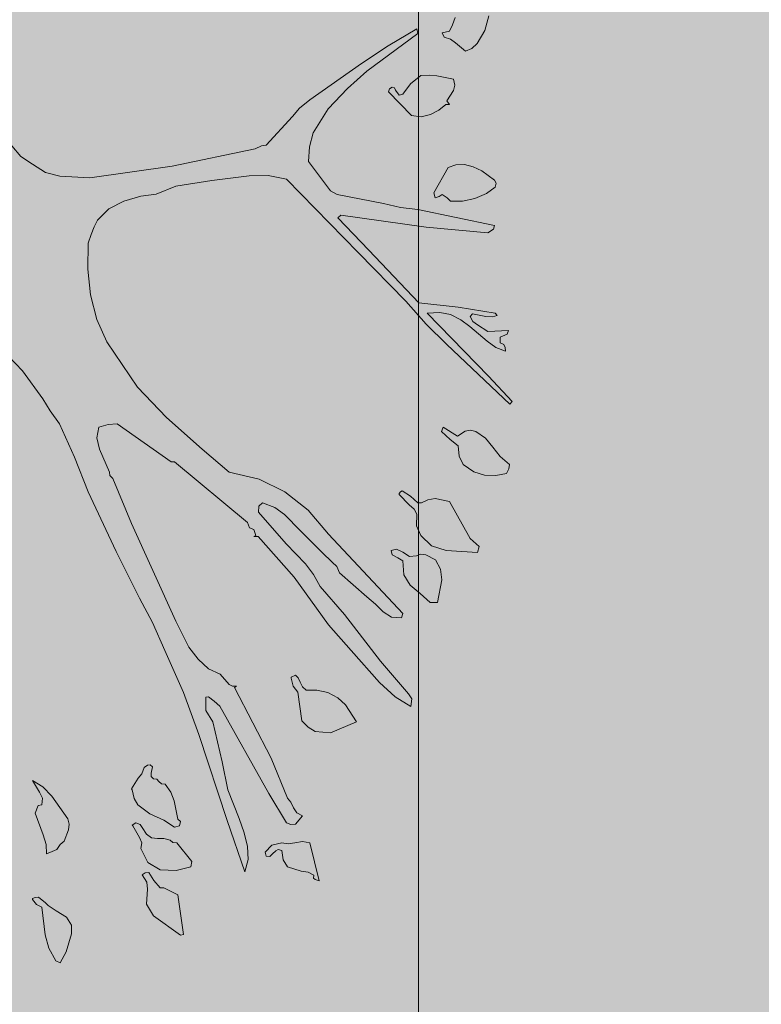
# Model space of a CAD drawing. Units: inches. Extents: x 84 to 1044, y -280 to 906.
# Tile 61 of 105: x 427 to 440, y 731 to 748. Entities that reach past the tile are written whole.
import ezdxf

# ---------------------------------------------------------------- set-up
doc = ezdxf.new("R2010")
doc.units = ezdxf.units.IN
for name, color, linetype, lineweight in [('A-ANNO-DIMS', 2, 'Continuous', 18), ('L-HRDS', 32, 'Continuous', 18), ('L-PLNT', 114, 'Continuous', 15)]:
    doc.layers.add(name, color=color, linetype=linetype, lineweight=lineweight)
doc.layers.add('L-PLNT-PATT', color=9, linetype='Continuous', lineweight=9, true_color=0xafd9aa)
doc.styles.get("Standard").update_dxf_attribs({"font": 'arial.ttf'})
doc.dimstyles.get("Standard").update_dxf_attribs({"dimtxt": 0.18, "dimasz": 0.18, "dimexe": 0.18, "dimexo": 0.0625, "dimgap": 0.09, "dimtad": 0, "dimtih": 1, "dimtoh": 1, "dimdec": 4, "dimzin": 0, "dimdsep": 46, "dimtxsty": 'Standard', "dimcen": 0.09, "dimadec": 0, "dimazin": 0, "dimtfac": 1, "dimtdec": 4, "dimtofl": 0, "dimtmove": 0, "dimatfit": 3, "dimfxl": 1, "dimtolj": 1, "dimtzin": 0, "dimarcsym": 0})

# ---------------------------------------------------------------- blocks, each defined once
blk = doc.blocks.new('A$C37E508DF')
for p, q in [((1.3455, 1.0934), (1.3485, 1.102)), ((1.3875, 1.1037), (1.3828, 1.087)), ((1.2713, 1.0694), (1.3044, 1.0887)), ((1.3044, 1.0887), (1.3057, 1.0835)), ((1.3421, 1.0861), (1.3455, 1.0934)), ((1.3057, 1.0835), (1.2469, 1.0402)), ((1.3335, 1.0844), (1.3421, 1.0861)), ((1.3361, 1.0793), (1.3335, 1.0844)), ((1.3434, 1.0771), (1.3361, 1.0793)), ((1.349, 1.0728), (1.3434, 1.0771)), ((1.3828, 1.087), (1.3738, 1.072)), ((1.2409, 1.0488), (1.2713, 1.0694)), ((1.3605, 1.063), (1.349, 1.0728)), ((1.3678, 1.0664), (1.3605, 1.063)), ((1.3738, 1.072), (1.3678, 1.0664)), ((1.1813, 1.0072), (1.2409, 1.0488)), ((1.2469, 1.0402), (1.2246, 1.0201)), ((1.2971, 1.0257), (1.3091, 1.0351)), ((1.3091, 1.0351), (1.3185, 1.0355)), ((1.3185, 1.0355), (1.3275, 1.0347)), ((1.3275, 1.0347), (1.3468, 1.0308)), ((1.2731, 1.0197), (1.2761, 1.0218)), ((1.2761, 1.0218), (1.2786, 1.0209)), ((1.2786, 1.0209), (1.2799, 1.0184)), ((1.2885, 1.0136), (1.2971, 1.0257)), ((1.3468, 1.0308), (1.3481, 1.0239)), ((1.3481, 1.0239), (1.3468, 1.018)), ((1.2246, 1.0201), (1.2023, 0.9969)), ((1.2718, 1.0162), (1.2731, 1.0197)), ((1.2984, 0.9892), (1.2718, 1.0162)), ((1.2799, 1.0184), (1.2842, 1.0124)), ((1.2842, 1.0124), (1.2885, 1.0136)), ((1.3468, 1.018), (1.3391, 1.0059)), ((1.1693, 0.9974), (1.1813, 1.0072)), ((1.3378, 1.0016), (1.3297, 0.9952)), ((1.3421, 1.0016), (1.3378, 1.0016)), ((1.3391, 1.0059), (1.3421, 1.0016)), ((1.1311, 0.9549), (1.1612, 0.9879)), ((1.1612, 0.9879), (1.1693, 0.9974)), ((1.2023, 0.9969), (1.1852, 0.9691)), ((1.3095, 0.9875), (1.2984, 0.9892)), ((1.3202, 0.9901), (1.3095, 0.9875)), ((1.3297, 0.9952), (1.3202, 0.9901)), ((1.1852, 0.9691), (1.1809, 0.9532)), ((0.8383, 0.954), (0.8486, 0.942)), ((1.1183, 0.9506), (1.1256, 0.954)), ((1.1256, 0.954), (1.1311, 0.9549)), ((1.1809, 0.9532), (1.1796, 0.936)), ((0.8486, 0.942), (0.8619, 0.933)), ((1.0227, 0.9309), (1.1183, 0.9506)), ((0.8619, 0.933), (0.8769, 0.9236)), ((0.9279, 0.9172), (1.0227, 0.9309)), ((1.1796, 0.936), (1.2049, 0.9022)), ((1.3404, 0.9292), (1.3494, 0.9322)), ((1.3494, 0.9322), (1.3592, 0.9326)), ((1.3592, 0.9326), (1.3695, 0.93)), ((1.3695, 0.93), (1.3794, 0.9253)), ((0.8769, 0.9236), (0.8936, 0.9193)), ((0.8936, 0.9193), (0.9279, 0.9172)), ((1.1114, 0.9198), (1.0685, 0.9142)), ((1.1333, 0.9202), (1.1114, 0.9198)), ((1.1543, 0.9159), (1.1333, 0.9202)), ((1.3241, 0.9), (1.3404, 0.9292)), ((1.3794, 0.9253), (1.394, 0.9146)), ((1.0269, 0.9077), (1.0042, 0.8987)), ((1.0685, 0.9142), (1.0269, 0.9077)), ((1.2371, 0.8314), (1.1543, 0.9159)), ((1.394, 0.9146), (1.3957, 0.9112)), ((1.3957, 0.9112), (1.3948, 0.9065)), ((0.9866, 0.8962), (0.9673, 0.8906)), ((1.0042, 0.8987), (0.9866, 0.8962)), ((1.2049, 0.9022), (1.2126, 0.8983)), ((1.2126, 0.8983), (1.2662, 0.8876)), ((1.3254, 0.8944), (1.3241, 0.9)), ((1.3301, 0.8957), (1.3254, 0.8944)), ((1.3335, 0.8983), (1.3301, 0.8957)), ((1.3395, 0.8944), (1.3335, 0.8983)), ((1.3846, 0.8992), (1.3713, 0.8936)), ((1.3948, 0.9065), (1.3846, 0.8992)), ((0.9673, 0.8906), (0.9498, 0.8816)), ((1.2662, 0.8876), (1.2855, 0.8833)), ((1.3434, 0.8906), (1.3395, 0.8944)), ((1.3571, 0.8906), (1.3434, 0.8906)), ((1.3713, 0.8936), (1.3571, 0.8906)), ((0.9498, 0.8816), (0.9369, 0.8687)), ((1.2169, 0.8743), (1.2135, 0.8713)), ((1.3151, 0.8606), (1.2169, 0.8743)), ((1.2855, 0.8833), (1.3057, 0.8807)), ((1.3057, 0.8807), (1.394, 0.8623)), ((0.9369, 0.8687), (0.933, 0.861)), ((1.2135, 0.8713), (1.2491, 0.834)), ((1.394, 0.8623), (1.3927, 0.8584)), ((0.9296, 0.852), (0.9262, 0.8421)), ((0.933, 0.861), (0.9296, 0.852)), ((1.3863, 0.8541), (1.3151, 0.8606)), ((1.3927, 0.8584), (1.3863, 0.8541)), ((0.9262, 0.8421), (0.9257, 0.8121)), ((1.2919, 0.7752), (1.2371, 0.8314)), ((1.2491, 0.834), (1.3069, 0.7735)), ((0.9257, 0.8121), (0.9287, 0.7825)), ((0.9287, 0.7825), (0.936, 0.7542)), ((1.3151, 0.7487), (1.2919, 0.7752)), ((1.3069, 0.7735), (1.352, 0.7684)), ((1.3309, 0.7624), (1.3164, 0.7615)), ((1.3164, 0.7615), (1.3871, 0.6891)), ((1.3434, 0.7598), (1.3309, 0.7624)), ((1.355, 0.7538), (1.3434, 0.7598)), ((1.352, 0.7684), (1.3948, 0.7615)), ((1.3687, 0.7607), (1.3657, 0.7577)), ((1.3841, 0.7577), (1.3687, 0.7607)), ((1.3948, 0.7615), (1.397, 0.759)), ((0.936, 0.7542), (0.9476, 0.7285)), ((1.3391, 0.7255), (1.3151, 0.7487)), ((1.3653, 0.7461), (1.355, 0.7538)), ((1.3657, 0.7577), (1.3691, 0.7521)), ((1.3691, 0.7521), (1.3743, 0.7482)), ((1.3743, 0.7482), (1.3863, 0.7405)), ((1.3914, 0.7572), (1.3841, 0.7577)), ((1.397, 0.759), (1.3914, 0.7572)), ((1.3854, 0.7294), (1.3653, 0.7461)), ((1.3863, 0.7405), (1.4099, 0.7414)), ((1.4086, 0.7375), (1.4004, 0.7337)), ((1.4099, 0.7414), (1.4086, 0.7375)), ((0.9476, 0.7285), (0.9828, 0.6762)), ((1.4116, 0.6569), (1.3391, 0.7255)), ((1.3953, 0.7221), (1.3854, 0.7294)), ((1.4004, 0.7337), (1.4004, 0.7272)), ((1.4004, 0.7272), (1.4047, 0.7255)), ((1.4047, 0.7255), (1.406, 0.7221)), ((1.4064, 0.7178), (1.3953, 0.7221)), ((1.406, 0.7221), (1.4064, 0.7178)), ((0.8503, 0.6951), (0.8344, 0.7122)), ((0.8739, 0.6629), (0.8503, 0.6951)), ((1.3871, 0.6891), (1.4141, 0.6599)), ((0.9828, 0.6762), (1.0162, 0.6415)), ((0.8824, 0.6492), (0.8739, 0.6629)), ((1.4141, 0.6599), (1.4116, 0.6569)), ((0.8932, 0.6342), (0.8824, 0.6492)), ((1.0162, 0.6415), (1.0574, 0.605)), ((0.9103, 0.5956), (0.8932, 0.6342)), ((0.9382, 0.6303), (0.936, 0.6179)), ((0.9493, 0.6333), (0.9382, 0.6303)), ((0.9596, 0.6342), (0.9493, 0.6333)), ((1.0218, 0.5904), (0.9596, 0.6342)), ((1.3327, 0.6252), (1.3348, 0.6303)), ((1.343, 0.6162), (1.3327, 0.6252)), ((1.3348, 0.6303), (1.3511, 0.62)), ((1.3511, 0.62), (1.3601, 0.6256)), ((1.3601, 0.6256), (1.3661, 0.6269)), ((1.3661, 0.6269), (1.3725, 0.6252)), ((1.3725, 0.6252), (1.3837, 0.6175)), ((0.936, 0.6179), (0.939, 0.605)), ((1.352, 0.6089), (1.343, 0.6162)), ((1.3837, 0.6175), (1.3918, 0.6072)), ((0.939, 0.605), (0.9506, 0.5784)), ((1.0574, 0.605), (1.0883, 0.5784)), ((1.3533, 0.5969), (1.352, 0.6089)), ((1.3918, 0.6072), (1.4004, 0.5964)), ((0.9262, 0.5557), (0.9103, 0.5956)), ((1.0256, 0.5904), (1.0218, 0.5904)), ((1.1097, 0.5205), (1.0256, 0.5904)), ((1.358, 0.5874), (1.3533, 0.5969)), ((1.4004, 0.5964), (1.4111, 0.5874)), ((0.9506, 0.5784), (0.951, 0.5746)), ((1.0883, 0.5784), (1.123, 0.5703)), ((1.37, 0.5789), (1.358, 0.5874)), ((1.3824, 0.575), (1.37, 0.5789)), ((1.4103, 0.5823), (1.4077, 0.5771)), ((1.4111, 0.5874), (1.4103, 0.5823)), ((0.951, 0.5746), (0.9545, 0.5711)), ((0.9545, 0.5711), (0.9759, 0.5193)), ((1.123, 0.5703), (1.1526, 0.5557)), ((1.3953, 0.5746), (1.3824, 0.575)), ((1.4077, 0.5771), (1.3953, 0.5746)), ((0.9583, 0.4871), (0.9262, 0.5557)), ((1.1526, 0.5557), (1.1792, 0.5347)), ((1.2842, 0.554), (1.2855, 0.5557)), ((1.2855, 0.5557), (1.2876, 0.557)), ((1.2876, 0.557), (1.2971, 0.551)), ((1.2842, 0.5527), (1.2842, 0.554)), ((1.2958, 0.5407), (1.2842, 0.5527)), ((1.2971, 0.551), (1.3057, 0.5433)), ((1.3099, 0.5433), (1.3172, 0.5467)), ((1.3172, 0.5467), (1.3254, 0.548)), ((1.3254, 0.548), (1.3421, 0.5446)), ((1.3421, 0.5446), (1.3657, 0.5021)), ((1.1226, 0.5394), (1.1221, 0.5325)), ((1.1268, 0.5433), (1.1226, 0.5394)), ((1.141, 0.5377), (1.1268, 0.5433)), ((1.1521, 0.5296), (1.141, 0.5377)), ((1.1792, 0.5347), (1.2027, 0.5072)), ((1.3014, 0.536), (1.2958, 0.5407)), ((1.3044, 0.53), (1.3014, 0.536)), ((1.3057, 0.5433), (1.3099, 0.5433)), ((1.1221, 0.5325), (1.1539, 0.4961)), ((1.1706, 0.5111), (1.1521, 0.5296)), ((1.3039, 0.5167), (1.3044, 0.53)), ((0.9759, 0.5193), (1.0269, 0.4069)), ((1.1118, 0.5145), (1.1097, 0.5205)), ((1.117, 0.5124), (1.1118, 0.5145)), ((1.1191, 0.5055), (1.117, 0.5124)), ((1.1955, 0.4858), (1.1706, 0.5111)), ((1.3091, 0.5055), (1.3039, 0.5167)), ((1.117, 0.5042), (1.1191, 0.5055)), ((1.1217, 0.5042), (1.117, 0.5042)), ((1.1633, 0.4575), (1.1217, 0.5042)), ((1.2027, 0.5072), (1.2426, 0.4644)), ((1.3215, 0.4935), (1.3091, 0.5055)), ((1.3657, 0.5021), (1.3764, 0.4927)), ((1.1539, 0.4961), (1.1762, 0.4729)), ((1.2748, 0.4884), (1.2812, 0.4897)), ((1.2761, 0.4832), (1.2748, 0.4884)), ((1.2812, 0.4897), (1.2885, 0.4862)), ((1.3382, 0.4884), (1.3215, 0.4935)), ((1.3743, 0.4858), (1.3382, 0.4884)), ((1.3764, 0.4927), (1.3743, 0.4858)), ((0.9853, 0.4335), (0.9583, 0.4871)), ((1.207, 0.4747), (1.1955, 0.4858)), ((1.2825, 0.4798), (1.2761, 0.4832)), ((1.2885, 0.4764), (1.2825, 0.4798)), ((1.2885, 0.4862), (1.2962, 0.4815)), ((1.2894, 0.4601), (1.2885, 0.4764)), ((1.2962, 0.4815), (1.3039, 0.482)), ((1.3039, 0.482), (1.3087, 0.4841)), ((1.3087, 0.4841), (1.3147, 0.4832)), ((1.3147, 0.4832), (1.3258, 0.4777)), ((1.3258, 0.4777), (1.3318, 0.4669)), ((1.1762, 0.4729), (1.1856, 0.4605)), ((1.2122, 0.47), (1.207, 0.4747)), ((1.2156, 0.4627), (1.2122, 0.47)), ((1.3318, 0.4669), (1.3331, 0.4545)), ((1.2027, 0.4026), (1.1633, 0.4575)), ((1.1856, 0.4605), (1.1933, 0.4468)), ((1.2469, 0.4348), (1.2156, 0.4627)), ((1.2426, 0.4644), (1.2885, 0.4159)), ((1.2967, 0.4485), (1.2894, 0.4601)), ((1.3331, 0.4545), (1.3284, 0.4284)), ((1.1933, 0.4468), (1.2212, 0.4146)), ((1.3082, 0.4386), (1.2967, 0.4485)), ((1.0003, 0.4052), (0.9853, 0.4335)), ((1.2568, 0.4266), (1.2469, 0.4348)), ((1.3198, 0.4284), (1.3082, 0.4386)), ((1.2658, 0.4176), (1.2568, 0.4266)), ((1.3284, 0.4284), (1.3198, 0.4284)), ((1.2212, 0.4146), (1.2628, 0.361)), ((1.2752, 0.4116), (1.2658, 0.4176)), ((1.2868, 0.4108), (1.2752, 0.4116)), ((1.2885, 0.4159), (1.2868, 0.4108)), ((1.0145, 0.373), (1.0003, 0.4052)), ((1.0269, 0.4069), (1.0419, 0.3769)), ((1.2289, 0.373), (1.2027, 0.4026)), ((1.0419, 0.3769), (1.0527, 0.3632)), ((1.0359, 0.3246), (1.0145, 0.373)), ((1.0527, 0.3632), (1.0647, 0.352)), ((1.2615, 0.3362), (1.2289, 0.373)), ((1.0647, 0.352), (1.078, 0.346)), ((1.2628, 0.361), (1.2949, 0.3233)), ((1.078, 0.346), (1.0883, 0.334)), ((1.1599, 0.3426), (1.1646, 0.3447)), ((1.1599, 0.3413), (1.1599, 0.3426)), ((1.162, 0.3319), (1.1599, 0.3413)), ((1.1646, 0.3447), (1.168, 0.3417)), ((1.168, 0.3417), (1.1702, 0.3366)), ((1.0883, 0.334), (1.0921, 0.3319)), ((1.0921, 0.3319), (1.0968, 0.3319)), ((1.0968, 0.3319), (1.0947, 0.3306)), ((1.0947, 0.3306), (1.1367, 0.2491)), ((1.1676, 0.325), (1.162, 0.3319)), ((1.1702, 0.3366), (1.1727, 0.3314)), ((1.1727, 0.3314), (1.177, 0.3276)), ((1.2795, 0.3199), (1.2615, 0.3362)), ((1.0535, 0.2766), (1.0359, 0.3246)), ((1.0647, 0.3199), (1.0617, 0.3194)), ((1.0617, 0.3194), (1.0617, 0.304)), ((1.0711, 0.3147), (1.0647, 0.3199)), ((1.1719, 0.292), (1.1676, 0.325)), ((1.177, 0.3276), (1.1895, 0.3276)), ((1.1895, 0.3276), (1.2019, 0.3246)), ((1.2019, 0.3246), (1.2135, 0.3186)), ((1.2135, 0.3186), (1.2225, 0.3104)), ((1.2975, 0.3087), (1.2795, 0.3199)), ((1.2949, 0.3233), (1.2988, 0.3173)), ((1.0775, 0.3092), (1.0711, 0.3147)), ((1.1341, 0.2084), (1.0775, 0.3092)), ((1.2225, 0.3104), (1.2349, 0.2911)), ((1.2988, 0.3173), (1.2975, 0.3087)), ((1.0617, 0.304), (1.0698, 0.2911)), ((1.0698, 0.2911), (1.0805, 0.2448)), ((1.1792, 0.2847), (1.1719, 0.292)), ((1.1873, 0.28), (1.1792, 0.2847)), ((1.2349, 0.2911), (1.2049, 0.2783)), ((1.0861, 0.1775), (1.0535, 0.2766)), ((1.2049, 0.2783), (1.1873, 0.28)), ((0.9879, 0.2311), (0.9905, 0.2384)), ((0.9905, 0.2384), (0.9943, 0.241)), ((0.9943, 0.241), (0.9973, 0.2414)), ((0.9973, 0.2414), (1.0003, 0.2393)), ((1.0003, 0.2393), (0.9986, 0.232)), ((1.0805, 0.2448), (1.087, 0.2127)), ((1.1367, 0.2491), (1.1556, 0.2032)), ((0.9836, 0.226), (0.9879, 0.2311)), ((0.9986, 0.232), (0.9986, 0.2281)), ((0.9986, 0.2281), (1.0012, 0.2255)), ((0.8619, 0.2234), (0.8739, 0.2161)), ((0.87, 0.2101), (0.8619, 0.2234)), ((0.8739, 0.2161), (0.8841, 0.2054)), ((0.9759, 0.214), (0.9836, 0.226)), ((1.0012, 0.2255), (1.0051, 0.2251)), ((1.0051, 0.2251), (1.0076, 0.2225)), ((1.0076, 0.2225), (1.0106, 0.2195)), ((1.0106, 0.2195), (1.0149, 0.2191)), ((1.0149, 0.2191), (1.0214, 0.2101)), ((0.8734, 0.2032), (0.87, 0.2101)), ((0.8841, 0.2054), (0.9026, 0.1792)), ((0.9768, 0.2127), (0.9759, 0.214)), ((0.9789, 0.2028), (0.9768, 0.2127)), ((1.0214, 0.2101), (1.0252, 0.2002)), ((1.087, 0.2127), (1.0998, 0.1797)), ((1.1543, 0.1749), (1.1341, 0.2084)), ((0.8649, 0.1857), (0.8687, 0.1947)), ((0.8687, 0.1947), (0.8726, 0.1955)), ((0.8726, 0.1955), (0.8734, 0.2032)), ((0.9832, 0.1955), (0.9789, 0.2028)), ((0.9969, 0.1852), (0.9832, 0.1955)), ((1.0252, 0.2002), (1.0295, 0.1788)), ((1.1556, 0.2032), (1.1594, 0.1985)), ((1.1594, 0.1985), (1.1624, 0.1921)), ((0.8743, 0.1608), (0.8649, 0.1857)), ((1.0132, 0.1779), (0.9969, 0.1852)), ((1.1624, 0.1921), (1.1663, 0.1861)), ((1.1727, 0.1827), (1.1646, 0.1732)), ((1.1663, 0.1861), (1.1727, 0.1827)), ((0.9026, 0.1792), (0.9043, 0.1732)), ((0.9043, 0.1732), (0.9035, 0.1668)), ((0.9768, 0.1719), (0.9811, 0.1749)), ((0.9776, 0.1711), (0.9768, 0.1719)), ((0.9853, 0.1578), (0.9776, 0.1711)), ((0.9811, 0.1749), (0.9858, 0.1728)), ((0.9858, 0.1728), (0.9884, 0.1694)), ((1.0256, 0.1698), (1.0132, 0.1779)), ((1.0312, 0.1711), (1.0256, 0.1698)), ((1.0295, 0.1788), (1.0325, 0.1762)), ((1.0325, 0.1762), (1.0312, 0.1711)), ((1.1063, 0.1183), (1.0861, 0.1775)), ((1.0998, 0.1797), (1.1058, 0.1634)), ((1.1594, 0.1728), (1.1543, 0.1749)), ((1.1646, 0.1732), (1.1594, 0.1728)), ((0.8777, 0.1496), (0.8743, 0.1608)), ((0.9035, 0.1668), (0.8983, 0.1535)), ((0.9884, 0.1694), (0.9931, 0.1616)), ((0.9931, 0.1616), (0.9991, 0.1574)), ((1.1058, 0.1634), (1.1097, 0.1475)), ((0.8781, 0.1389), (0.8777, 0.1496)), ((0.894, 0.1496), (0.8902, 0.1441)), ((0.8983, 0.1535), (0.894, 0.1496)), ((0.9879, 0.1518), (0.9853, 0.1578)), ((0.9866, 0.1453), (0.9879, 0.1518)), ((0.9991, 0.1574), (1.0059, 0.1565)), ((1.0059, 0.1565), (1.0132, 0.1565)), ((1.0132, 0.1565), (1.0205, 0.1548)), ((1.0205, 0.1548), (1.0235, 0.1522)), ((1.0235, 0.1522), (1.0282, 0.1518)), ((1.0282, 0.1518), (1.0454, 0.1303)), ((1.1097, 0.1475), (1.1101, 0.1325)), ((1.1298, 0.1411), (1.1376, 0.1492)), ((1.1376, 0.1492), (1.1491, 0.1518)), ((1.1491, 0.1518), (1.1564, 0.1505)), ((1.1564, 0.1505), (1.1642, 0.1518)), ((1.1642, 0.1518), (1.1727, 0.1531)), ((1.1727, 0.1531), (1.1813, 0.1518)), ((1.1813, 0.1518), (1.192, 0.108)), ((0.8846, 0.1419), (0.8781, 0.1389)), ((0.8902, 0.1441), (0.8846, 0.1419)), ((0.9948, 0.1291), (0.9866, 0.1453)), ((1.1311, 0.1364), (1.1298, 0.1411)), ((1.1354, 0.1359), (1.1311, 0.1364)), ((1.1384, 0.1389), (1.1354, 0.1359)), ((1.1423, 0.1423), (1.1384, 0.1389)), ((1.1449, 0.1441), (1.1423, 0.1423)), ((1.1491, 0.1428), (1.1449, 0.1441)), ((1.1504, 0.132), (1.1491, 0.1428)), ((1.0089, 0.1205), (0.9948, 0.1291)), ((1.0454, 0.1303), (1.0441, 0.1239)), ((1.1101, 0.1325), (1.1063, 0.1183)), ((1.1556, 0.1239), (1.1504, 0.132)), ((0.9884, 0.1149), (0.9918, 0.117)), ((0.9935, 0.1063), (0.9884, 0.1149)), ((0.9918, 0.117), (0.9961, 0.1175)), ((0.9961, 0.1175), (1.0016, 0.1085)), ((1.0274, 0.12), (1.0089, 0.1205)), ((1.0441, 0.1239), (1.0274, 0.12)), ((1.1714, 0.1192), (1.1556, 0.1239)), ((1.1792, 0.1179), (1.1714, 0.1192)), ((1.186, 0.1145), (1.1792, 0.1179)), ((1.1856, 0.111), (1.186, 0.1145)), ((0.9943, 0.0982), (0.9935, 0.1063)), ((1.0016, 0.1085), (1.0089, 0.0999)), ((1.1873, 0.1093), (1.1856, 0.111)), ((1.192, 0.108), (1.1873, 0.1093)), ((0.9931, 0.081), (0.9943, 0.0982)), ((1.0089, 0.0999), (1.0132, 0.0999)), ((1.0132, 0.0999), (1.0295, 0.0917)), ((1.0295, 0.0917), (1.0359, 0.0463)), ((0.8619, 0.0875), (0.8649, 0.0887)), ((0.8619, 0.0866), (0.8619, 0.0875)), ((0.8666, 0.0806), (0.8619, 0.0866)), ((0.8649, 0.0887), (0.8691, 0.0892)), ((0.8726, 0.0776), (0.8666, 0.0806)), ((0.8691, 0.0892), (0.8769, 0.0827)), ((0.8769, 0.0827), (0.8799, 0.0797)), ((0.8799, 0.0797), (0.8893, 0.0733)), ((1.0012, 0.0677), (0.9931, 0.081)), ((0.8764, 0.0459), (0.8726, 0.0776)), ((0.8893, 0.0733), (0.9013, 0.066)), ((0.9013, 0.066), (0.9069, 0.057)), ((0.9069, 0.057), (0.9069, 0.0471)), ((1.0325, 0.0454), (1.0012, 0.0677)), ((0.8807, 0.0304), (0.8764, 0.0459)), ((0.9069, 0.0471), (0.9009, 0.0261)), ((1.0359, 0.0463), (1.0325, 0.0454)), ((0.8889, 0.0159), (0.8807, 0.0304)), ((0.9009, 0.0261), (0.894, 0.0137)), ((0.894, 0.0137), (0.8889, 0.0159))]:
    blk.add_line(p, q)
blk = doc.blocks.new('*D62')
at = {"layer": 'A-ANNO-DIMS', "color": 0, "lineweight": -2, "transparency": 16777216}
for p, q in [((203.179, 709.183), (203.179, 905.9)), ((896.074, 400.183), (896.074, 905.9)), ((203.359, 905.72), (549.232, 905.72)), ((895.894, 905.72), (550.021, 905.72))]:
    blk.add_line(p, q, dxfattribs=at)
at = {"layer": 'A-ANNO-DIMS', "color": 0, "transparency": 16777216}
for points in [[(203.359, 905.75), (203.359, 905.69), (203.179, 905.72)], [(895.894, 905.75), (895.894, 905.69), (896.074, 905.72)]]:
    blk.add_solid(points, dxfattribs=at)
at = {"layer": 'Defpoints', "color": 0, "transparency": 16777216}
for p in [(896.074, 905.72), (203.179, 709.12), (896.074, 400.12)]:
    blk.add_point(p, dxfattribs=at)
at = {"layer": 'A-ANNO-DIMS', "color": 0, "transparency": 16777216, "insert": (549.627, 905.72), "char_height": 0.18, "attachment_point": 5}
blk.add_mtext('\\A1;692.9', dxfattribs=at)

msp = doc.modelspace()

# ---------------------------------------------------------------- hatches: boundary and pattern name
at = {"layer": 'L-PLNT-PATT', "transparency": 33554597}
h = msp.add_hatch(color=256, dxfattribs=at)
h.dxf.hatch_style = 1
h.paths.add_polyline_path([(434.074, 769.12), (386.074, 769.12), (386.074, 709.12), (434.074, 709.12)])
h.paths.add_polyline_path([(896.074, 847.12), (434.074, 847.12), (434.074, 769.12), (434.074, 709.12), (470.074, 709.12), (506.074, 709.12), (572.074, 709.12), (608.074, 709.12), (698.074, 709.12), (770.074, 709.12), (833.074, 709.12), (896.074, 709.12)])
h.paths.add_polyline_path([(983.074, 847.12), (896.074, 847.12), (896.074, 709.12), (896.074, 547.12), (932.074, 547.12), (983.074, 547.12)])
h.paths.add_polyline_path([(983.074, 547.12), (932.074, 547.12), (932.074, 265.12), (983.074, 265.12)])
h.paths.add_polyline_path([(203.179, 646.12), (203.179, 709.12), (203.179, 745.12), (143.179, 745.12), (143.179, 271.12), (203.179, 271.12), (203.179, 274.12), (203.179, 310.12), (203.179, 574.12)])

# ---------------------------------------------------------------- linework, layer by layer
at = {"layer": 'L-HRDS'}
msp.add_line((434.074, 769.12), (434.074, 709.12), dxfattribs=at)

# ---------------------------------------------------------------- block references
at = {"layer": 'L-PLNT', "xscale": 15.19586232982809, "yscale": 15.19586232982809, "zscale": 15.19586232982809}
msp.add_blockref('A$C37E508DF', (414.225, 731.356), dxfattribs=at)

# ---------------------------------------------------------------- dimensions: what is measured, and where the dimension line sits
at = {"layer": 'A-ANNO-DIMS'}
dim = msp.add_linear_dim(base=(896.074, 905.72), p1=(203.179, 709.12), p2=(896.074, 400.12), dimstyle='Standard', override={"dimdec": 1, "dimlfac": 1, "dimrnd": 0, "dimzin": 0, "dimdsep": 46, "dimlunit": 2}, dxfattribs=at)
dim.commit()
dim.dimension.update_dxf_attribs({"geometry": '*D62', "text_midpoint": (549.627, 905.72)})

doc.saveas('drawing.dxf')
